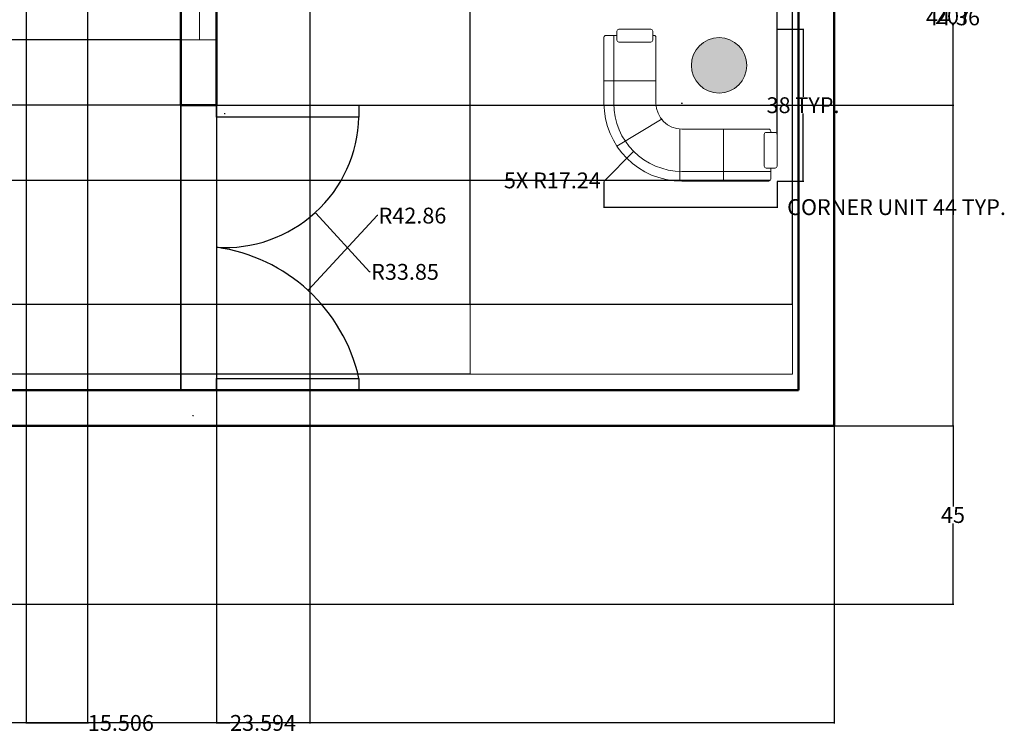
# Model space of a CAD drawing. Units: inches. Extents: x 1454 to 2136, y 626 to 1213.
# Tile 21 of 23: x 1887 to 2136, y 626 to 806. Entities that reach past the tile are written whole.
import ezdxf

# ---------------------------------------------------------------- set-up
doc = ezdxf.new("R2010")
doc.units = ezdxf.units.IN
doc.header["$MEASUREMENT"] = 0
for name, color, linetype, lineweight in [('A-ANNO-DIMS', 2, 'Continuous', 18), ('A-DOOR', 3, 'Continuous', 25), ('A-FURN', 9, 'Continuous', 18), ('A-FURN-PATT', 252, 'Continuous', 13), ('A-GLAZ', 4, 'Continuous', 18), ('A-WALL', 7, 'Continuous', 50), ('sofa', 4, 'Continuous', 18)]:
    doc.layers.add(name, color=color, linetype=linetype, lineweight=lineweight)
doc.styles.get("Standard").update_dxf_attribs({"font": 'arial.ttf'})
doc.dimstyles.get("Standard").update_dxf_attribs({"dimtxt": 4, "dimasz": 0.18, "dimexe": 0.18, "dimexo": 0.0625, "dimgap": 0.09, "dimtad": 0, "dimtih": 1, "dimtoh": 1, "dimdec": 0, "dimrnd": 6, "dimzin": 0, "dimdsep": 46, "dimlunit": 3, "dimtxsty": 'Standard', "dimcen": 0.09, "dimadec": 0, "dimazin": 0, "dimtfac": 1, "dimtdec": 0, "dimtofl": 0, "dimtmove": 0, "dimatfit": 3, "dimfxl": 1, "dimtolj": 1, "dimtzin": 0, "dimarcsym": 0})

# ---------------------------------------------------------------- blocks, each defined once
blk = doc.blocks.new('A$C42183DBB')
for p, q in [((0.144, 1.661), (0.144, 1.562)), ((0.166, 1.682), (0.518, 1.682)), ((0.54, 1.661), (0.54, 1.562)), ((0, 1.592), (0, 0.864)), ((0.022, 1.614), (0.144, 1.614)), ((0.108, 1.614), (0.108, 0.864)), ((0.166, 1.541), (0.518, 1.541)), ((0.54, 1.614), (0.554, 1.614)), ((0.576, 1.592), (0.576, 0.864)), ((0, 1.11), (0.576, 1.11)), ((0.643, 0.69), (0.142, 0.389)), ((0.84, 0.576), (0.84, 0)), ((0.864, 0.576), (1.826, 0.576)), ((1.322, 0.576), (1.322, 0)), ((1.848, 0.54), (1.848, 0.554)), ((1.775, 0.166), (1.775, 0.518)), ((1.895, 0.54), (1.797, 0.54)), ((1.917, 0.166), (1.917, 0.518)), ((1.895, 0.144), (1.797, 0.144)), ((1.848, 0.022), (1.848, 0.144)), ((0.864, 0.108), (1.848, 0.108)), ((0.864, 0), (1.826, 0))]:
    blk.add_line(p, q)
for centre, radius, start, end in [((0.166, 1.661), 0.0216, 90, 180), ((0.518, 1.661), 0.0216, 0, 90), ((0.022, 1.592), 0.0216, 90, 180), ((0.166, 1.562), 0.0216, 180, 270), ((0.518, 1.562), 0.0216, 270, 0), ((0.554, 1.592), 0.0216, 0, 90), ((0.864, 0.864), 0.864, 180, 270), ((0.864, 0.864), 0.756, 180, 270), ((0.864, 0.864), 0.288, 180, 270), ((1.826, 0.554), 0.0216, 0, 90), ((1.797, 0.518), 0.0216, 90, 180), ((1.895, 0.518), 0.0216, 0, 90), ((1.797, 0.166), 0.0216, 180, 270), ((1.895, 0.166), 0.0216, 270, 0), ((1.826, 0.022), 0.0216, 270, 0)]:
    blk.add_arc(centre, radius, start, end)
blk = doc.blocks.new('WIN-34_84')
blk.add_line((34.84, 4.31), (0, 4.31))
blk.add_lwpolyline([(34.84, 0), (0, 0), (0, 9), (34.84, 9)], close=True)
blk = doc.blocks.new('DOOR-LEAF-36')
blk.add_lwpolyline([(-36, 3), (0, 3), (0, 0), (-36, 0)], close=True)
blk = doc.blocks.new('*D9')
at = {"layer": 'A-ANNO-DIMS', "color": 0, "lineweight": -2, "transparency": 16777216}
for p, q in [((2034.43, 765.03), (2034.43, 758.36)), ((2078.14, 765.03), (2078.14, 758.36)), ((2034.61, 758.54), (2077.96, 758.54)), ((2078.14, 758.54), (2078.32, 758.54))]:
    blk.add_line(p, q, dxfattribs=at)
at = {"layer": 'A-ANNO-DIMS', "color": 0, "transparency": 16777216}
for points in [[(2034.61, 758.57), (2034.61, 758.51), (2034.43, 758.54)], [(2077.96, 758.57), (2077.96, 758.51), (2078.14, 758.54)]]:
    blk.add_solid(points, dxfattribs=at)
at = {"layer": 'Defpoints', "color": 0, "transparency": 16777216}
for p in [(2034.43, 765.1), (2078.14, 765.1), (2078.14, 758.54)]:
    blk.add_point(p, dxfattribs=at)
at = {"layer": 'A-ANNO-DIMS', "color": 0, "transparency": 16777216, "insert": (2108.3, 758.54), "char_height": 4, "attachment_point": 5}
blk.add_mtext('\\A1;CORNER UNIT 44 TYP.', dxfattribs=at)
blk = doc.blocks.new('*D10')
at = {"layer": 'A-ANNO-DIMS', "color": 0, "lineweight": -2, "transparency": 16777216}
for p, q in [((2078.2, 803.46), (2084.87, 803.46)), ((2084.69, 803.28), (2084.69, 786.41)), ((2084.69, 765.28), (2084.69, 782.15)), ((2078.2, 765.1), (2084.87, 765.1))]:
    blk.add_line(p, q, dxfattribs=at)
at = {"layer": 'A-ANNO-DIMS', "color": 0, "transparency": 16777216}
for points in [[(2084.66, 803.28), (2084.72, 803.28), (2084.69, 803.46)], [(2084.66, 765.28), (2084.72, 765.28), (2084.69, 765.1)]]:
    blk.add_solid(points, dxfattribs=at)
at = {"layer": 'Defpoints', "color": 0, "transparency": 16777216}
for p in [(2078.14, 803.46), (2084.69, 803.46), (2078.14, 765.1)]:
    blk.add_point(p, dxfattribs=at)
at = {"layer": 'A-ANNO-DIMS', "color": 0, "transparency": 16777216, "insert": (2084.69, 784.28), "char_height": 4, "attachment_point": 5}
blk.add_mtext('\\A1;38 TYP.', dxfattribs=at)
blk = doc.blocks.new('*D27')
at = {"layer": 'A-ANNO-DIMS', "color": 0, "lineweight": -2, "transparency": 16777216}
for p, q in [((2092.56, 703.22), (2092.56, 628.1)), ((1492.56, 658.22), (1492.56, 628.1)), ((1492.74, 628.28), (1788.04, 628.28)), ((2092.38, 628.28), (1797.07, 628.28))]:
    blk.add_line(p, q, dxfattribs=at)
at = {"layer": 'A-ANNO-DIMS', "color": 0, "transparency": 16777216}
for points in [[(1492.74, 628.31), (1492.74, 628.25), (1492.56, 628.28)], [(2092.38, 628.31), (2092.38, 628.25), (2092.56, 628.28)]]:
    blk.add_solid(points, dxfattribs=at)
at = {"layer": 'Defpoints', "color": 0, "transparency": 16777216}
for p in [(2092.56, 703.28), (1492.56, 658.28), (2092.56, 628.28)]:
    blk.add_point(p, dxfattribs=at)
at = {"layer": 'A-ANNO-DIMS', "color": 0, "transparency": 16777216, "insert": (1792.56, 628.28), "char_height": 4, "attachment_point": 5}
blk.add_mtext('\\A1;600', dxfattribs=at)
blk = doc.blocks.new('*D35')
at = {"layer": 'A-ANNO-DIMS', "color": 0, "lineweight": -2, "transparency": 16777216}
for p, q in [((2092.62, 910.28), (2122.74, 910.28)), ((2122.56, 910.1), (2122.56, 808.91)), ((2122.56, 703.46), (2122.56, 804.65)), ((2092.62, 703.28), (2122.74, 703.28))]:
    blk.add_line(p, q, dxfattribs=at)
at = {"layer": 'A-ANNO-DIMS', "color": 0, "transparency": 16777216}
for points in [[(2122.53, 910.1), (2122.59, 910.1), (2122.56, 910.28)], [(2122.53, 703.46), (2122.59, 703.46), (2122.56, 703.28)]]:
    blk.add_solid(points, dxfattribs=at)
at = {"layer": 'Defpoints', "color": 0, "transparency": 16777216}
for p in [(2092.56, 910.28), (2092.56, 703.28), (2122.56, 703.28)]:
    blk.add_point(p, dxfattribs=at)
at = {"layer": 'A-ANNO-DIMS', "color": 0, "transparency": 16777216, "insert": (2122.56, 806.78), "char_height": 4, "attachment_point": 5}
blk.add_mtext('\\A1;207', dxfattribs=at)
blk = doc.blocks.new('*D37')
at = {"layer": 'A-ANNO-DIMS', "color": 0, "lineweight": -2, "transparency": 16777216}
for p, q in [((1774.56, 712.34), (1774.56, 1210.46)), ((1774.74, 1210.28), (1846.74, 1210.28)), ((1927.38, 1210.28), (1855.38, 1210.28)), ((1927.56, 712.34), (1927.56, 1210.46))]:
    blk.add_line(p, q, dxfattribs=at)
at = {"layer": 'A-ANNO-DIMS', "color": 0, "transparency": 16777216}
for points in [[(1774.74, 1210.31), (1774.74, 1210.25), (1774.56, 1210.28)], [(1927.38, 1210.31), (1927.38, 1210.25), (1927.56, 1210.28)]]:
    blk.add_solid(points, dxfattribs=at)
at = {"layer": 'Defpoints', "color": 0, "transparency": 16777216}
for p in [(1927.56, 1210.28), (1774.56, 712.28), (1927.56, 712.28)]:
    blk.add_point(p, dxfattribs=at)
at = {"layer": 'A-ANNO-DIMS', "color": 0, "transparency": 16777216, "insert": (1851.06, 1210.28), "char_height": 4, "attachment_point": 5}
blk.add_mtext('\\A1;153', dxfattribs=at)
blk = doc.blocks.new('*D38')
at = {"layer": 'A-ANNO-DIMS', "color": 0, "lineweight": -2, "transparency": 16777216}
for p, q in [((1783.62, 703.28), (2122.74, 703.28)), ((2122.56, 703.1), (2122.56, 682.91)), ((2122.56, 658.46), (2122.56, 678.66)), ((1783.62, 658.28), (2122.74, 658.28))]:
    blk.add_line(p, q, dxfattribs=at)
at = {"layer": 'A-ANNO-DIMS', "color": 0, "transparency": 16777216}
for points in [[(2122.53, 703.1), (2122.59, 703.1), (2122.56, 703.28)], [(2122.53, 658.46), (2122.59, 658.46), (2122.56, 658.28)]]:
    blk.add_solid(points, dxfattribs=at)
at = {"layer": 'Defpoints', "color": 0, "transparency": 16777216}
for p in [(1783.56, 703.28), (2122.56, 703.28), (1783.56, 658.28)]:
    blk.add_point(p, dxfattribs=at)
at = {"layer": 'A-ANNO-DIMS', "color": 0, "transparency": 16777216, "insert": (2122.56, 680.78), "char_height": 4, "attachment_point": 5}
blk.add_mtext('\\A1;45', dxfattribs=at)
blk = doc.blocks.new('*D52')
at = {"layer": 'A-ANNO-DIMS', "color": 0, "lineweight": -2, "transparency": 16777216}
for p, q in [((1927.57, 800.77), (1462.37, 800.77)), ((1462.55, 800.59), (1462.55, 794.66)), ((1462.55, 784.46), (1462.55, 790.4)), ((1927.49, 784.28), (1462.37, 784.28))]:
    blk.add_line(p, q, dxfattribs=at)
at = {"layer": 'A-ANNO-DIMS', "color": 0, "transparency": 16777216}
for points in [[(1462.52, 800.59), (1462.58, 800.59), (1462.55, 800.77)], [(1462.52, 784.46), (1462.58, 784.46), (1462.55, 784.28)]]:
    blk.add_solid(points, dxfattribs=at)
at = {"layer": 'Defpoints', "color": 0, "transparency": 16777216}
for p in [(1462.55, 800.77), (1927.64, 800.77), (1927.56, 784.28)]:
    blk.add_point(p, dxfattribs=at)
at = {"layer": 'A-ANNO-DIMS', "color": 0, "transparency": 16777216, "insert": (1462.55, 792.53), "char_height": 4, "attachment_point": 5}
blk.add_mtext('\\A1;16.49', dxfattribs=at)
blk = doc.blocks.new('*D61')
at = {"layer": 'A-ANNO-DIMS', "color": 0, "lineweight": -2, "transparency": 16777216}
for p, q in [((1888.56, 1126.22), (1888.56, 628.1)), ((1904.06, 1126.38), (1904.06, 628.1)), ((1888.74, 628.28), (1903.88, 628.28)), ((1904.06, 628.28), (1904.24, 628.28))]:
    blk.add_line(p, q, dxfattribs=at)
at = {"layer": 'A-ANNO-DIMS', "color": 0, "transparency": 16777216}
for points in [[(1888.74, 628.31), (1888.74, 628.25), (1888.56, 628.28)], [(1903.88, 628.31), (1903.88, 628.25), (1904.06, 628.28)]]:
    blk.add_solid(points, dxfattribs=at)
at = {"layer": 'Defpoints', "color": 0, "transparency": 16777216}
for p in [(1888.56, 1126.28), (1904.06, 1126.44), (1904.06, 628.28)]:
    blk.add_point(p, dxfattribs=at)
at = {"layer": 'A-ANNO-DIMS', "color": 0, "transparency": 16777216, "insert": (1912.45, 628.28), "char_height": 4, "attachment_point": 5}
blk.add_mtext('\\A1;15.506', dxfattribs=at)
blk = doc.blocks.new('*D63')
at = {"layer": 'A-ANNO-DIMS', "color": 0, "lineweight": -2, "transparency": 16777216}
for p, q in [((2000.63, 733.98), (2000.63, 1210.46)), ((2000.81, 1210.28), (2034.88, 1210.28)), ((2081.86, 1210.28), (2047.79, 1210.28)), ((2082.04, 733.98), (2082.04, 1210.46))]:
    blk.add_line(p, q, dxfattribs=at)
at = {"layer": 'A-ANNO-DIMS', "color": 0, "transparency": 16777216}
for points in [[(2000.81, 1210.31), (2000.81, 1210.25), (2000.63, 1210.28)], [(2081.86, 1210.31), (2081.86, 1210.25), (2082.04, 1210.28)]]:
    blk.add_solid(points, dxfattribs=at)
at = {"layer": 'Defpoints', "color": 0, "transparency": 16777216}
for p in [(2082.04, 1210.28), (2000.63, 733.92), (2082.04, 733.92)]:
    blk.add_point(p, dxfattribs=at)
at = {"layer": 'A-ANNO-DIMS', "color": 0, "transparency": 16777216, "insert": (2041.33, 1210.28), "char_height": 4, "attachment_point": 5}
blk.add_mtext('\\A1;81.41', dxfattribs=at)
blk = doc.blocks.new('*D64')
at = {"layer": 'A-ANNO-DIMS', "color": 0, "lineweight": -2, "transparency": 16777216}
for p, q in [((2000.57, 733.92), (1462.37, 733.92)), ((1462.55, 733.74), (1462.55, 727.25)), ((1462.55, 716.5), (1462.55, 722.99)), ((2000.57, 716.32), (1462.37, 716.32))]:
    blk.add_line(p, q, dxfattribs=at)
at = {"layer": 'A-ANNO-DIMS', "color": 0, "transparency": 16777216}
for points in [[(1462.52, 733.74), (1462.58, 733.74), (1462.55, 733.92)], [(1462.52, 716.5), (1462.58, 716.5), (1462.55, 716.32)]]:
    blk.add_solid(points, dxfattribs=at)
at = {"layer": 'Defpoints', "color": 0, "transparency": 16777216}
for p in [(1462.55, 733.92), (2000.63, 733.92), (2000.63, 716.32)]:
    blk.add_point(p, dxfattribs=at)
at = {"layer": 'A-ANNO-DIMS', "color": 0, "transparency": 16777216, "insert": (1462.55, 725.12), "char_height": 4, "attachment_point": 5}
blk.add_mtext('\\A1;17.604', dxfattribs=at)
blk = doc.blocks.new('*D84')
at = {"layer": 'A-ANNO-DIMS', "color": 0, "lineweight": -2, "transparency": 16777216}
for p, q in [((1958.1, 828.64), (2122.74, 828.64)), ((2122.56, 828.46), (2122.56, 808.6)), ((2122.56, 784.46), (2122.56, 804.33)), ((1936.62, 784.28), (2122.74, 784.28))]:
    blk.add_line(p, q, dxfattribs=at)
at = {"layer": 'A-ANNO-DIMS', "color": 0, "transparency": 16777216}
for points in [[(2122.53, 828.46), (2122.59, 828.46), (2122.56, 828.64)], [(2122.53, 784.46), (2122.59, 784.46), (2122.56, 784.28)]]:
    blk.add_solid(points, dxfattribs=at)
at = {"layer": 'Defpoints', "color": 0, "transparency": 16777216}
for p in [(1958.04, 828.64), (2122.56, 828.64), (1936.56, 784.28)]:
    blk.add_point(p, dxfattribs=at)
at = {"layer": 'A-ANNO-DIMS', "color": 0, "transparency": 16777216, "insert": (2122.56, 806.46), "char_height": 4, "attachment_point": 5}
blk.add_mtext('\\A1;44.36', dxfattribs=at)
blk = doc.blocks.new('*D85')
at = {"layer": 'A-ANNO-DIMS', "color": 0, "lineweight": -2, "transparency": 16777216}
for p, q in [((1936.56, 901.22), (1936.56, 628.1)), ((1960.15, 891.55), (1960.15, 628.1)), ((1936.74, 628.28), (1939.93, 628.28)), ((1959.97, 628.28), (1956.77, 628.28))]:
    blk.add_line(p, q, dxfattribs=at)
at = {"layer": 'A-ANNO-DIMS', "color": 0, "transparency": 16777216}
for points in [[(1936.74, 628.31), (1936.74, 628.25), (1936.56, 628.28)], [(1959.97, 628.31), (1959.97, 628.25), (1960.15, 628.28)]]:
    blk.add_solid(points, dxfattribs=at)
at = {"layer": 'Defpoints', "color": 0, "transparency": 16777216}
for p in [(1936.56, 901.28), (1960.15, 891.61), (1960.15, 628.28)]:
    blk.add_point(p, dxfattribs=at)
at = {"layer": 'A-ANNO-DIMS', "color": 0, "transparency": 16777216, "insert": (1948.35, 628.28), "char_height": 4, "attachment_point": 5}
blk.add_mtext('\\A1;23.594', dxfattribs=at)
blk = doc.blocks.new('*D86')
at = {"layer": 'A-ANNO-DIMS', "color": 0, "lineweight": -2, "transparency": 16777216}
for p, q in [((2078.14, 1210.28), (2077.96, 1210.28)), ((2078.14, 776.98), (2078.14, 1210.46)), ((2083.38, 1210.28), (2078.32, 1210.28)), ((2083.56, 712.34), (2083.56, 1210.46))]:
    blk.add_line(p, q, dxfattribs=at)
at = {"layer": 'A-ANNO-DIMS', "color": 0, "transparency": 16777216}
for points in [[(2078.32, 1210.31), (2078.32, 1210.25), (2078.14, 1210.28)], [(2083.38, 1210.31), (2083.38, 1210.25), (2083.56, 1210.28)]]:
    blk.add_solid(points, dxfattribs=at)
at = {"layer": 'Defpoints', "color": 0, "transparency": 16777216}
for p in [(2078.14, 1210.28), (2078.14, 776.92), (2083.56, 712.28)]:
    blk.add_point(p, dxfattribs=at)
at = {"layer": 'A-ANNO-DIMS', "color": 0, "transparency": 16777216, "insert": (2072.69, 1210.28), "char_height": 4, "attachment_point": 5}
blk.add_mtext('\\A1;5.42', dxfattribs=at)
blk = doc.blocks.new('*D87')
at = {"layer": 'A-ANNO-DIMS', "color": 0, "lineweight": -2, "transparency": 16777216}
for p, q in [((2076.36, 765.24), (1462.37, 765.24)), ((1462.55, 765.06), (1462.55, 751.71)), ((1462.55, 734.1), (1462.55, 747.45)), ((2081.97, 733.92), (1462.37, 733.92))]:
    blk.add_line(p, q, dxfattribs=at)
at = {"layer": 'A-ANNO-DIMS', "color": 0, "transparency": 16777216}
for points in [[(1462.52, 765.06), (1462.58, 765.06), (1462.55, 765.24)], [(1462.52, 734.1), (1462.58, 734.1), (1462.55, 733.92)]]:
    blk.add_solid(points, dxfattribs=at)
at = {"layer": 'Defpoints', "color": 0, "transparency": 16777216}
for p in [(1462.55, 765.24), (2076.42, 765.24), (2082.04, 733.92)]:
    blk.add_point(p, dxfattribs=at)
at = {"layer": 'A-ANNO-DIMS', "color": 0, "transparency": 16777216, "insert": (1462.55, 749.58), "char_height": 4, "attachment_point": 5}
blk.add_mtext('\\A1;31.32', dxfattribs=at)
blk = doc.blocks.new('*D94')
at = {"layer": 'A-ANNO-DIMS', "color": 0, "lineweight": -2, "transparency": 16777216}
for p, q in [((1977.15, 756.4), (1959.86, 737.61)), ((1977.33, 756.4), (1977.15, 756.4)), ((1930.64, 705.93), (1930.82, 705.93)), ((1930.73, 705.84), (1930.73, 706.02))]:
    blk.add_line(p, q, dxfattribs=at)
at = {"layer": 'A-ANNO-DIMS', "color": 0, "transparency": 16777216}
blk.add_solid([(1959.84, 737.63), (1959.89, 737.59), (1959.74, 737.48)], dxfattribs=at)
at = {"layer": 'Defpoints', "color": 0, "transparency": 16777216}
for p in [(1959.74, 737.48), (1930.73, 705.93)]:
    blk.add_point(p, dxfattribs=at)
at = {"layer": 'A-ANNO-DIMS', "color": 0, "transparency": 16777216, "insert": (1986.08, 756.4), "char_height": 4, "attachment_point": 5}
blk.add_mtext('\\A1;R42.86', dxfattribs=at)
blk = doc.blocks.new('*D96')
at = {"layer": 'A-ANNO-DIMS', "color": 0, "lineweight": -2, "transparency": 16777216}
for p, q in [((1938.62, 782.17), (1938.8, 782.17)), ((1938.71, 782.08), (1938.71, 782.26)), ((1975.25, 742.19), (1961.67, 757.05)), ((1975.43, 742.19), (1975.25, 742.19))]:
    blk.add_line(p, q, dxfattribs=at)
at = {"layer": 'A-ANNO-DIMS', "color": 0, "transparency": 16777216}
blk.add_solid([(1961.69, 757.07), (1961.65, 757.03), (1961.55, 757.18)], dxfattribs=at)
at = {"layer": 'Defpoints', "color": 0, "transparency": 16777216}
for p in [(1938.71, 782.17), (1961.55, 757.18)]:
    blk.add_point(p, dxfattribs=at)
at = {"layer": 'A-ANNO-DIMS', "color": 0, "transparency": 16777216, "insert": (1984.2, 742.19), "char_height": 4, "attachment_point": 5}
blk.add_mtext('\\A1;R33.85', dxfattribs=at)
blk = doc.blocks.new('*D100')
at = {"layer": 'A-ANNO-DIMS', "color": 0, "lineweight": -2, "transparency": 16777216}
for p, q in [((2054.04, 784.8), (2054.22, 784.8)), ((2054.13, 784.71), (2054.13, 784.89)), ((2034.63, 765.29), (2041.81, 772.48)), ((2034.45, 765.29), (2034.63, 765.29))]:
    blk.add_line(p, q, dxfattribs=at)
at = {"layer": 'A-ANNO-DIMS', "color": 0, "transparency": 16777216}
blk.add_solid([(2041.79, 772.5), (2041.83, 772.46), (2041.94, 772.61)], dxfattribs=at)
at = {"layer": 'Defpoints', "color": 0, "transparency": 16777216}
for p in [(2054.13, 784.8), (2041.94, 772.61)]:
    blk.add_point(p, dxfattribs=at)
at = {"layer": 'A-ANNO-DIMS', "color": 0, "transparency": 16777216, "insert": (2021.4, 765.29), "char_height": 4, "attachment_point": 5}
blk.add_mtext('\\A1;5X R17.24', dxfattribs=at)

msp = doc.modelspace()

# ---------------------------------------------------------------- hatches: boundary and pattern name
at = {"layer": 'A-FURN-PATT'}
h = msp.add_hatch(dxfattribs=at)
h.set_pattern_fill('ESCHER', color=256)
h.paths.add_polyline_path([(1511.3761, 923.7174, 1), (1525.379, 923.7174, 1)])
h.paths.add_polyline_path([(1525.379, 816.0542, 1), (1511.3761, 816.0542, 1)])
h.paths.add_polyline_path([(1525.379, 712.7345, 1), (1511.3761, 712.7345, 1)])
h.paths.add_polyline_path([(2070.5057, 794.3402, 1), (2056.5027, 794.3402, 1)])
h.paths.add_polyline_path([(2005.868, 1014.5578, 1), (1991.8651, 1014.5578, 1)])
h.paths.add_polyline_path([(1994.0647, 1066.7584, 1), (2008.0677, 1066.7584, 1)])
h.paths.add_polyline_path([(1919.5492, 1065.3848, 1), (1933.5521, 1065.3848, 1)])
h.paths.add_polyline_path([(1936.8517, 1013.7336, 1), (1922.8488, 1013.7336, 1)])
h.paths.add_polyline_path([(1824.6062, 1109.1557, 1), (1838.6091, 1109.1557, 1)])

# ---------------------------------------------------------------- linework, layer by layer
at = {"layer": 'A-DOOR'}
for p, q in [((1927.5563, 784.2825), (1927.5563, 712.2825)), ((1936.5563, 784.2825), (1936.5563, 712.2825))]:
    msp.add_line(p, q, dxfattribs=at)
for centre, radius, start, end in [((1938.715, 782.1731), 33.8531, 266.344046, 358.492422), ((1930.7311, 705.9281), 42.8585, 12.606915, 82.188308)]:
    msp.add_arc(centre, radius, start, end, dxfattribs=at)
at = {"layer": 'A-FURN'}
msp.add_lwpolyline([(2000.6276, 733.9205), (2082.0362, 733.9205), (2082.0362, 716.3161), (2000.6276, 716.3161)], close=True, dxfattribs=at)
msp.add_circle((2063.5042, 794.3402), 7.0015, dxfattribs=at)
at = {"layer": 'A-WALL'}
for p, q in [((1927.5563, 784.2825), (1927.5563, 910.2825)), ((2092.5563, 703.2825), (2092.5563, 910.2825)), ((1936.5563, 784.2825), (1936.5563, 901.2825)), ((2083.5563, 712.2825), (2083.5563, 901.2825)), ((1936.5563, 784.2825), (1927.5563, 784.2825)), ((2083.5563, 712.2825), (1774.5563, 712.2825)), ((2092.5563, 703.2825), (1783.5563, 703.2825))]:
    msp.add_line(p, q, dxfattribs=at)

# ---------------------------------------------------------------- block references
at = {"layer": 'A-DOOR'}
for p in [(1972.5563, 781.2825), (1972.5563, 712.2825)]:
    msp.add_blockref('DOOR-LEAF-36', p, dxfattribs=at)
at = {"layer": 'A-GLAZ', "rotation": 89.9999999999993}
msp.add_blockref('WIN-34_84', (1936.6352, 800.7734), dxfattribs=at)
at = {"layer": 'sofa', "xscale": 22.80350778510874, "yscale": 22.80350778510874, "zscale": 22.80350778510874}
msp.add_blockref('A$C42183DBB', (2034.4274, 765.0966), dxfattribs=at)

# ---------------------------------------------------------------- dimensions: what is measured, and where the dimension line sits
at = {"layer": 'A-ANNO-DIMS'}
for base, p1, p2, override, picture, middle in [((1927.5563, 1210.2845), (1774.5563, 712.2825), (1927.5563, 712.2825), {"dimdec": 0, "dimlfac": 1, "dimrnd": 0, "dimzin": 0, "dimdsep": 46, "dimlunit": 2}, '*D37', (1851.0563, 1210.2845)), ((2082.0362, 1210.2845), (2000.6276, 733.9205), (2082.0362, 733.9205), {"dimdec": 2, "dimlfac": 1, "dimrnd": 0, "dimzin": 0, "dimdsep": 46, "dimlunit": 2}, '*D63', (2041.3319, 1210.2845)), ((2078.1364, 1210.2845), (2083.5563, 712.2825), (2078.1364, 776.9179), {"dimdec": 2, "dimlfac": 1, "dimrnd": 0, "dimzin": 0, "dimdsep": 46, "dimlunit": 2}, '*D86', (2072.6917, 1210.2845)), ((1904.0619, 628.2805), (1888.5563, 1126.2825), (1904.0619, 1126.439), {"dimdec": 3, "dimlfac": 1, "dimrnd": 0, "dimzin": 0, "dimdsep": 46, "dimlunit": 2}, '*D61', (1912.4452, 628.2805)), ((1960.1503, 628.2805), (1936.5563, 901.2825), (1960.1503, 891.6137), {"dimdec": 3, "dimlfac": 1, "dimrnd": 0, "dimzin": 0, "dimdsep": 46, "dimlunit": 2}, '*D85', (1948.3533, 628.2805)), ((2092.5563, 628.2805), (1492.5563, 658.2825), (2092.5563, 703.2825), {"dimdec": 0, "dimlfac": 1, "dimrnd": 0, "dimzin": 0, "dimdsep": 46, "dimlunit": 2}, '*D27', (1792.5563, 628.2805))]:
    dim = msp.add_linear_dim(base=base, p1=p1, p2=p2, dimstyle='Standard', override=override, dxfattribs=at)
    dim.commit()
    dim.dimension.update_dxf_attribs({"geometry": picture, "text_midpoint": middle})
for base, p1, p2, override, picture, middle in [((2122.5583, 703.2825), (2092.5563, 910.2825), (2092.5563, 703.2825), {"dimdec": 0, "dimlfac": 1, "dimrnd": 0, "dimzin": 0, "dimdsep": 46, "dimlunit": 2}, '*D35', (2122.5583, 806.7825)), ((2122.5583, 828.6443), (1936.5563, 784.2825), (1958.0422, 828.6443), {"dimdec": 2, "dimlfac": 1, "dimrnd": 0, "dimzin": 0, "dimdsep": 46, "dimlunit": 2}, '*D84', (2122.5583, 806.4634)), ((1462.5543, 800.7734), (1927.5563, 784.2825), (1927.6352, 800.7734), {"dimdec": 2, "dimlfac": 1, "dimrnd": 0, "dimzin": 0, "dimdsep": 46, "dimlunit": 2}, '*D52', (1462.5543, 792.5279)), ((1462.5543, 765.2409), (2082.0362, 733.9205), (2076.4223, 765.2409), {"dimdec": 2, "dimlfac": 1, "dimrnd": 0, "dimzin": 0, "dimdsep": 46, "dimlunit": 2}, '*D87', (1462.5543, 749.5807)), ((1462.5543, 733.9205), (2000.6276, 716.3161), (2000.6276, 733.9205), {"dimdec": 3, "dimlfac": 1, "dimrnd": 0, "dimzin": 0, "dimdsep": 46, "dimlunit": 2}, '*D64', (1462.5543, 725.1183)), ((2122.5583, 703.2825), (1783.5563, 658.2825), (1783.5563, 703.2825), {"dimdec": 0, "dimlfac": 1, "dimrnd": 0, "dimzin": 0, "dimdsep": 46, "dimlunit": 2}, '*D38', (2122.5583, 680.7825))]:
    dim = msp.add_linear_dim(base=base, p1=p1, p2=p2, angle=90, dimstyle='Standard', override=override, dxfattribs=at)
    dim.commit()
    dim.dimension.update_dxf_attribs({"geometry": picture, "text_midpoint": middle})
dim = msp.add_linear_dim(base=(2084.6927, 803.461), p1=(2078.1364, 765.0966), p2=(2078.1364, 803.461), angle=90, text='<> TYP.', dimstyle='Standard', override={"dimdec": 0, "dimlfac": 1, "dimrnd": 0, "dimzin": 0, "dimdsep": 46, "dimlunit": 2}, dxfattribs=at)
dim.commit()
dim.dimension.update_dxf_attribs({"geometry": '*D10', "text_midpoint": (2084.6927, 784.2788)})
dim = msp.add_radius_dim(center=(2054.1296, 784.7988), mpoint=(2041.9396, 772.6086), text='5X <>', dimstyle='Standard', override={"dimdec": 2, "dimlfac": 1, "dimrnd": 0, "dimzin": 0, "dimdsep": 46, "dimlunit": 2}, dxfattribs=at)
dim.commit()
dim.dimension.update_dxf_attribs({"geometry": '*D100', "text_midpoint": (2021.4033, 765.2945), "dimtype": 164})
for center, mpoint, picture, middle in [((1938.715, 782.1731), (1961.5499, 757.1811), '*D96', (1984.1988, 742.186)), ((1930.7311, 705.9281), (1959.7421, 737.4751), '*D94', (1986.0804, 756.4033))]:
    dim = msp.add_radius_dim(center=center, mpoint=mpoint, dimstyle='Standard', override={"dimdec": 2, "dimlfac": 1, "dimrnd": 0, "dimzin": 0, "dimdsep": 46, "dimlunit": 2}, dxfattribs=at)
    dim.commit()
    dim.dimension.update_dxf_attribs({"geometry": picture, "text_midpoint": middle, "dimtype": 164})
dim = msp.add_linear_dim(base=(2078.1364, 758.5402), p1=(2034.4274, 765.0966), p2=(2078.1364, 765.0966), text='CORNER UNIT <> TYP.', dimstyle='Standard', override={"dimdec": 0, "dimlfac": 1, "dimrnd": 0, "dimzin": 0, "dimdsep": 46, "dimlunit": 2}, dxfattribs=at)
dim.commit()
dim.dimension.update_dxf_attribs({"geometry": '*D9', "text_midpoint": (2108.2972, 758.5402)})

doc.saveas('drawing.dxf')
